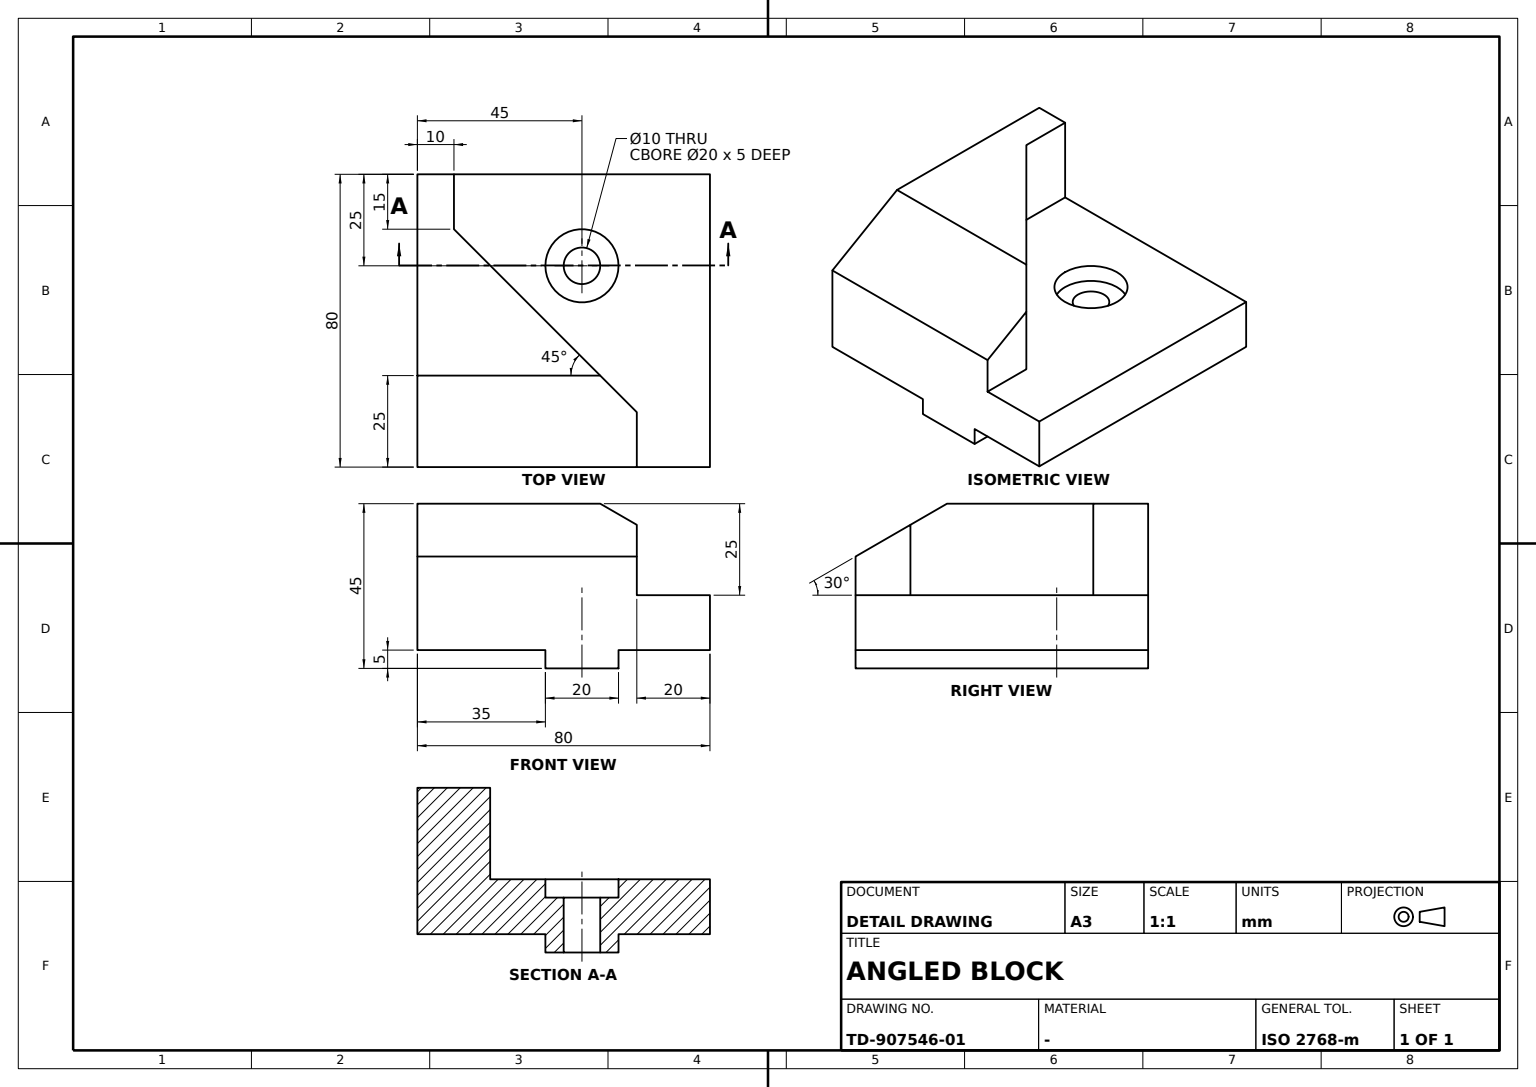
CATIA V5 part; units mm, degrees
sketch "Sketch1" plane through (0, 0, 0) normal (0, 1, 0) x (-1, 0, 0)
  line L0 (0, 0) -> (0, 40)
  line L1 (0, 40) -> (-10, 40)
  line L2 (-10, 40) -> (-10, 15)
  line L3 (-10, 15) -> (-80, 15)
  line L4 (-80, 15) -> (-80, 0)
  point P0 (-80, 0)
  line L5 (-80, 0) -> (-55, 0)
  line L6 (-55, 0) -> (-55, -5)
  line L7 (-55, -5) -> (-35, -5)
  line L8 (-35, -5) -> (-35, 0)
  point P1 (-35, 0)
  line L9 (-35, 0) -> (0, 0)
  dimension "length L7" = 20
  dimension "distance y axis L4" = 80
  dimension "length L4" = 15
  dimension "length L1" = 10
  dimension "length L0" = 40
  dimension "distance L7 L3" = 20
  dimension "length L5" = 25
  constraint vertical L0 y-axis
  constraint vertical L2 y-axis
  constraint vertical L4 y-axis
  constraint vertical L6 y-axis
  constraint vertical L8 y-axis
  constraint horizontal L1 x-axis
  constraint horizontal L3 x-axis
  constraint horizontal L5 x-axis
  constraint horizontal L7 x-axis
  constraint horizontal L9 x-axis
  constraint coincidence P0 x-axis
  constraint coincidence P1 x-axis
extrude "Pad1" add sketch "Sketch1" along normal mid plane 80
sketch "Sketch2" plane through (0, 0, 40) normal (0, 0, 1) x (0, -1, 0)
  line L0 (-25, 10) -> (40, 10)
  line L1 (40, 10) -> (40, 0)
  line L2 (40, 0) -> (-25, 0)
  line L3 (-25, 0) -> (-25, 10)
  line L4 (-40, 0) -> (-40, 10) construction
  line L5 (-40, 10) -> (40, 10) construction
  line L6 (40, 0) -> (40, 10) construction
  dimension "distance L3 L4" = 15
  constraint horizontal L0 x-axis
  constraint horizontal L2 x-axis
  constraint vertical L1 y-axis
  constraint vertical L3 y-axis
  constraint coincidence L0 L5
  constraint coincidence L1 L6
extrude "Pocket1" cut sketch "Sketch2" against normal blind 25
sketch "Sketch3" plane through (0, 0, 15) normal (0, 0, 1) x (0, -1, 0)
  line L0 (-25, 10) -> (40, 75)
  line L1 (-25, 10) -> (-25, 0)
  line L2 (-25, 0) -> (40, 0)
  point P0 (40, 0)
  point P1 (40, 60)
  line L3 (-25, 10) -> (-25, 0) construction
  line L4 (-25, 0) -> (40, 0) construction
  line L5 (40, 0) -> (40, 75)
  line L6 (40, 10) -> (40, 80) construction
  dimension "D1" = 45
  dimension "length L1" = 10
  constraint vertical L1 y-axis
  constraint vertical L5 y-axis
  constraint coincidence P0 x-axis
  constraint coincidence L1 L3
  constraint coincidence L2 L4
  constraint coincidence L5 L6
extrude "Pad2" add sketch "Sketch3" along normal blind 25
sketch "Sketch4" plane through (0, 0, 40) normal (0, 0, 1) x (1, 0, 0)
  point P0 (0, -39.8808)
  point P1 (60, -40)
  line L0 (80, 40) -> (80, -40) construction
  line L1 (60, -40) -> (60, -20.3962)
  line L2 (60, -20.3962) -> (80, -20.3962)
  line L3 (80, -20.3962) -> (80, -40)
  line L4 (80, -40) -> (60, -40)
  line L5 (80, 40) -> (80, -40) construction
  line L6 (0, -40) -> (75, -40) construction
  dimension "distance P1 L0" = 20
  constraint coincidence P0 y-axis
  constraint coincidence L3 L5
  constraint coincidence L4 L6
  constraint vertical L1 y-axis
  constraint vertical L3 y-axis
  constraint horizontal L2 x-axis
  constraint horizontal L4 x-axis
extrude "Pocket2" cut sketch "Sketch4" against normal blind 25
sketch "Sketch5" plane through (0, 0, 0) normal (-1, 0, 0) x (0, -1, 0)
  line L0 (15, 40) -> (40, 40)
  line L1 (40, 40) -> (40, 25.5662)
  line L2 (40, 25.5662) -> (15, 40)
  line L3 (40, 0) -> (40, 40) construction
  line L4 (-40, 40) -> (40, 40) construction
  dimension "length L0" = 25
  dimension "angle L0 L2" = 30
  constraint horizontal L0 x-axis
  constraint vertical L1 y-axis
  constraint coincidence L1 L3
  constraint coincidence L0 L4
extrude "Pocket3" cut sketch "Sketch5" against normal up to next
sketch "Sketch6" plane through (53.9445, 11.3763, 15) normal (0, 0, 1) x (1, 0, 0)
  point P0 (-8.9445, 3.6237)
  line L0 (26.0555, 28.6237) -> (26.0555, -51.3763) construction
  line L1 (-43.9445, 28.6237) -> (26.0555, 28.6237) construction
  dimension "distance P0 L0" = 35
  dimension "distance P0 L1" = 25
hole "Hole1" at (45, 15, 15) direction (0, 0, -1) diameter 20 depth 5
sketch "Sketch7" plane through (39.2678, 8.3576, 10) normal (0, 0, 1) x (1, 0, 0)
  point P0 (5.7322, 6.6424)
  circle A0 centre (5.7322, 6.6424) radius 10 construction
  constraint concentricity A0 P0
hole "Hole2" at (45, 15, 10) direction (0, 0, -1) diameter 10 end up to next
properties part number "catia 30"
